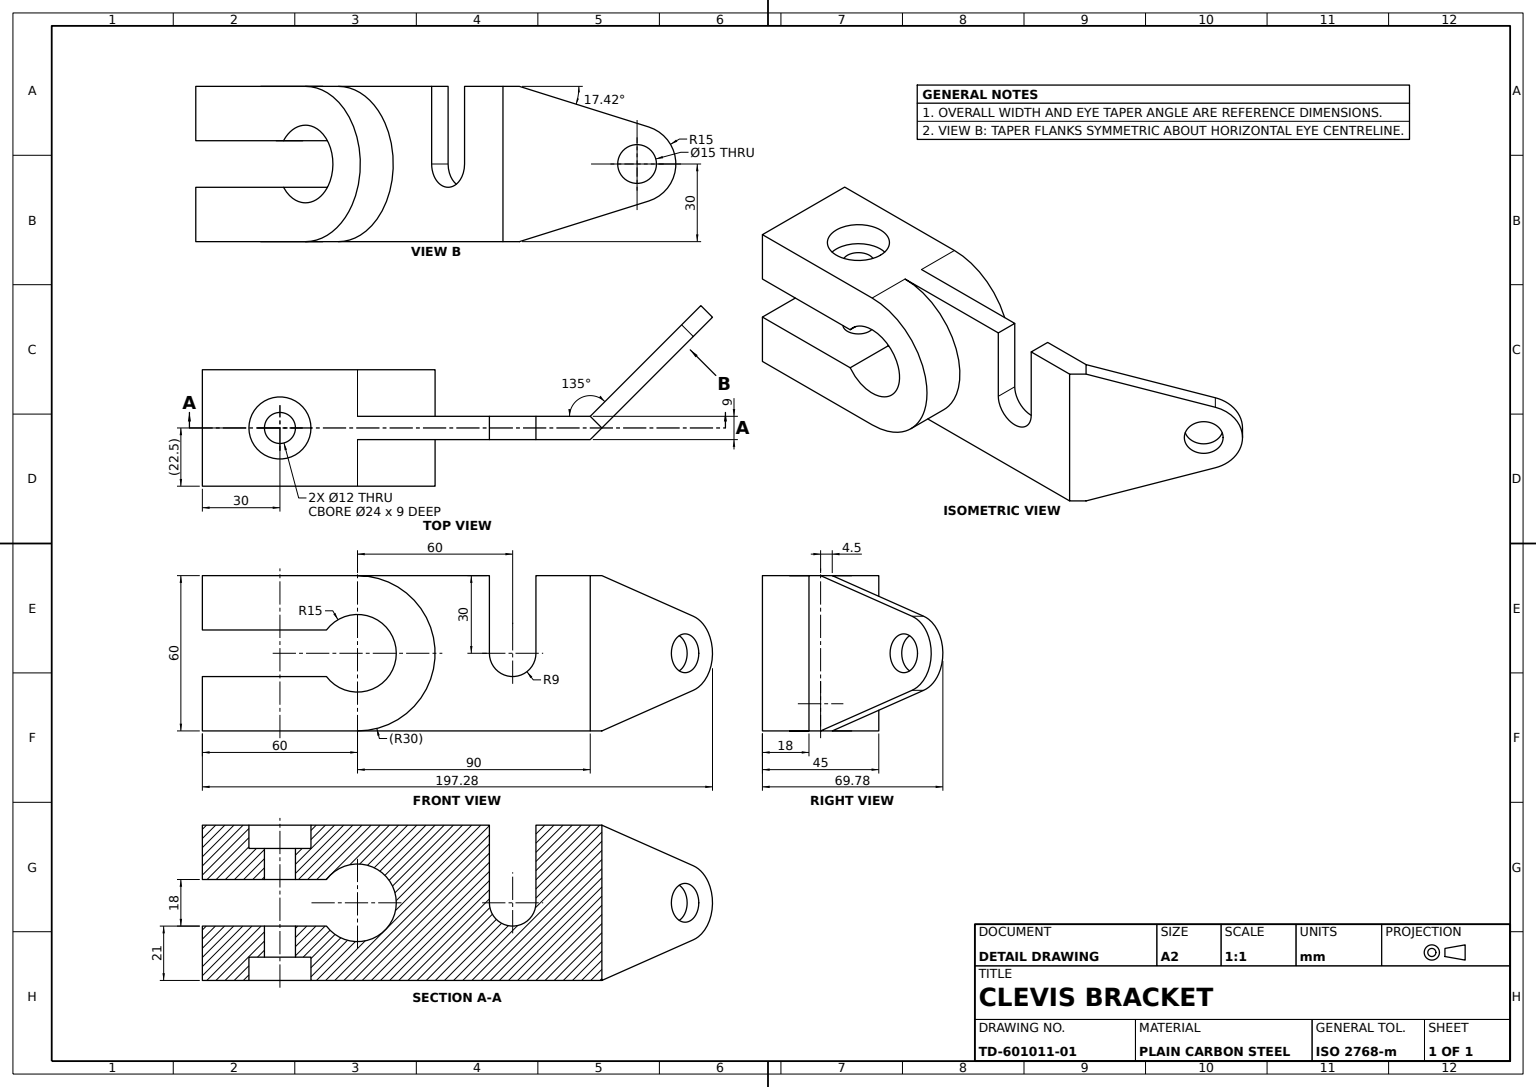
from build123d import *

# Parameters (mm, degrees)
CLEVIS_BLOCK_DEPTH         = 22.5
COUNTERBORE_SKETCH_R       = 12
PIN_HOLE_COUNTERBORE_DEPTH = 9
PIN_HOLE_SKETCH_R          = 6
PIN_HOLE_12_DEPTH          = 21
MOUNTING_ARM_DEPTH         = 30
ARM_CLEARANCE_CUT_DEPTH    = 30
EYE_PROFILE_CUT_DEPTH      = 30
EYE_BORE_SKETCH_R          = 7.5
EYE_BORE_DEPTH             = 30
RELIEF_SLOT_CUT_DEPTH      = 148.549271396
RELIEF_SLOT_CUT_DEPTH_BACK = 148.549271396


with BuildPart() as part:
    # Clevis Block Sketch → Clevis Block (new, symmetric)
    with BuildSketch(Plane.XY):
        with BuildLine():
            Line((0, -30), (-60, -30))
            Line((-60, -30), (-60, -9))
            Line((-60, -9), (-28.618176043, -9))
            Line((-28.618176043, -9), (-12, -9))
            ThreePointArc((-12, -9), (15, 0), (-12, 9))
            Line((-12, 9), (-28.618176043, 9))
            Line((-28.618176043, 9), (-60, 9))
            Line((-60, 9), (-60, 30))
            Line((-60, 30), (0, 30))
            ThreePointArc((0, 30), (30, 0), (0, -30))
        make_face()
    extrude(amount=CLEVIS_BLOCK_DEPTH, both=True)

    # Counterbore Sketch → Pin Hole Counterbore (cut)
    with BuildSketch(Plane(origin=(0, 30, 0), x_dir=(1, 0, 0), z_dir=(0, 1, 0))):
        with Locations(Location((-30, 0, 0), (0, 0, 180))):
            Circle(COUNTERBORE_SKETCH_R)
    pin_hole_counterbore = extrude(amount=-PIN_HOLE_COUNTERBORE_DEPTH, mode=Mode.SUBTRACT)

    # Pin Hole Sketch → Pin Hole Ø12 (cut)
    with BuildSketch(Plane(origin=(0, 30, 0), x_dir=(1, 0, 0), z_dir=(0, 1, 0))):
        with Locations(Location((-30, 0, 0), (0, 0, 180))):
            Circle(PIN_HOLE_SKETCH_R)
    pin_hole_12 = extrude(amount=-PIN_HOLE_12_DEPTH, mode=Mode.SUBTRACT)

    # Counterbore Mirror: Pin Hole Counterbore across plane
    add(pin_hole_counterbore.mirror(Plane.ZX), mode=Mode.SUBTRACT)

    # Pin Hole Mirror: Pin Hole Ø12 across plane
    add(pin_hole_12.mirror(Plane.ZX), mode=Mode.SUBTRACT)

    # Mounting Arm Sketch → Mounting Arm (add, symmetric)
    with BuildSketch(Plane(origin=(0, 0, 0), x_dir=(1, 0, 0), z_dir=(0, 1, 0))):
        Polygon((0, -4.5), (90, -4.5), (137.279960262, 42.779960262), (132.779960262, 47.279960262), (90, 4.5), (0, 4.5), align=None)
    extrude(amount=MOUNTING_ARM_DEPTH, both=True)

    # Arm Clearance Cut Sketch → Arm Clearance Cut (cut, symmetric)
    with BuildSketch(Plane(origin=(0, 0, -4.5), x_dir=(-1, 0, 0), z_dir=(0, 0, -1))):
        with BuildLine():
            Line((-51, 21), (-51, 30))
            Line((-51, 30), (-60, 30))
            Line((-60, 30), (-69, 30))
            Line((-69, 30), (-69, 0))
            ThreePointArc((-69, 0), (-60, -9), (-51, 0))
            Line((-51, 0), (-51, 21))
        make_face()
    extrude(amount=ARM_CLEARANCE_CUT_DEPTH, both=True, mode=Mode.SUBTRACT)

    # Eye Profile Cut Sketch → Eye Profile Cut (cut, symmetric)
    with BuildSketch(Plane(origin=(42.75, 0, 42.75), x_dir=(-0.7071067811865513, 0, 0.7071067811865437), z_dir=(-0.7071067811865437, 0, -0.7071067811865513))):
        with BuildLine():
            Line((-127.321590822, 30), (-127.321590822, 0))
            ThreePointArc((-127.321590822, 0), (-124.412282123, 8.87779161), (-116.812899639, 14.311818372))
            Line((-116.812899639, 14.311818372), (-66.821590822, 30))
            Line((-66.821590822, 30), (-127.321590822, 30))
        make_face()
        with BuildLine():
            ThreePointArc((-116.812899639, -14.311818372), (-124.412282123, -8.87779161), (-127.321590822, 0))
            Line((-127.321590822, 0), (-127.321590822, -30))
            Line((-127.321590822, -30), (-66.821590822, -30))
            Line((-66.821590822, -30), (-116.812899639, -14.311818372))
        make_face()
    extrude(amount=EYE_PROFILE_CUT_DEPTH, both=True, mode=Mode.SUBTRACT)

    # Eye Bore Sketch → Eye Bore (cut, symmetric)
    with BuildSketch(Plane(origin=(42.75, 0, 42.75), x_dir=(-0.7071067811865513, 0, 0.7071067811865437), z_dir=(-0.7071067811865437, 0, -0.7071067811865513))):
        with Locations((-112.321590822, 0)):
            Circle(EYE_BORE_SKETCH_R)
    extrude(amount=EYE_BORE_DEPTH, both=True, mode=Mode.SUBTRACT)

    # Relief Slot Sketch → Relief Slot Cut (cut, two sides: drawn at the far end of the back side and taken through both)
    with BuildSketch(Plane(origin=(0, 0, -22.5), x_dir=(-1, 0, 0), z_dir=(0, 0, -1)).offset(-RELIEF_SLOT_CUT_DEPTH_BACK)):
        with BuildLine():
            Line((0, 15), (0, -15))
            ThreePointArc((0, -15), (-15, 0), (0, 15))
        make_face()
    extrude(amount=RELIEF_SLOT_CUT_DEPTH + RELIEF_SLOT_CUT_DEPTH_BACK, mode=Mode.SUBTRACT)


solid = part.part
